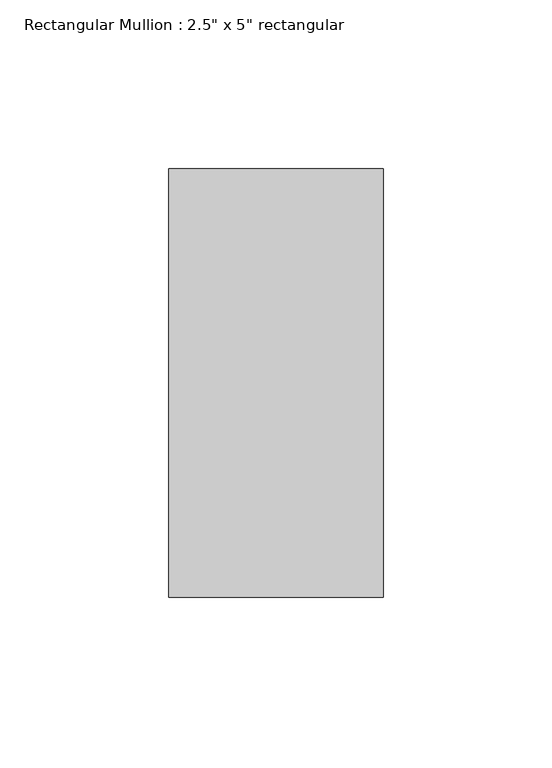
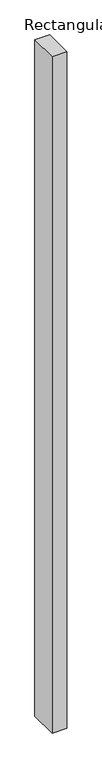
"""IFC4 building model written with IfcOpenShell, lengths in millimetres: member geometry."""

from ifc_helpers import new_model, si_unit, frame, origin, place, context, project, spatial, polyline, outline, extrude, source, transform, mapped, element, save


def member_eaba9652(model_context):
    return source(origin(), model_context, "Body", "SweptSolid", [
        extrude(outline(polyline([(31.75, 63.5), (31.75, -63.5), (-31.75, -63.5), (-31.75, 63.5), (31.75, 63.5)])), frame((0.0, 0.0, -3048.0), z_axis=(0.0, 0.0, 1.0), x_axis=(1.0, 0.0, 0.0)), (0.0, 0.0, 1.0), 3048.0),
    ])


if __name__ == "__main__":
    model = new_model("IFC4")
    model_context = context("Model", 3, world=origin())
    ifc_project = project(units=[si_unit("LENGTHUNIT", "METRE", prefix="MILLI")], contexts=[model_context])
    site = spatial("IfcSite", under=ifc_project)
    building = spatial("IfcBuilding", under=site)
    placement = place(None, origin())
    member_shape = member_eaba9652(model_context)
    element("IfcMember", 1, ObjectType="Rectangular Mullion : 2.5\" x 5\" rectangular", at=placement, inside=building, context=model_context, shape_type="MappedRepresentation", body=[
        mapped(member_shape, transform((0.0, 0.0, 0.0), x_axis=(1.0, 0.0, 0.0), y_axis=(0.0, 1.0, 0.0), z_axis=(0.0, 0.0, 1.0))),
    ])
    save(model, "model.ifc")

# Revit data of these elements
# Type "Rectangular Mullion : 2.5\" x 5\" rectangular"
#   built-in parameter 1007304 = 0.416667 (stored number, unit not read)
#   built-in parameter 1007301 = 0.104167 (stored number, unit not read)
#   built-in parameter 1007300 = 0.104167 (stored number, unit not read)
# Element 1 (IfcMember, "Rectangular Mullion : 2.5\" x 5\" rectangular")
#   Materials on its faces: "Iron, Ductile"
# Materials
#   "Iron, Ductile": class "Metal", colour RGB 0 0 0, transparency 0, Description = "Ductile cast iron", Cost = 0
